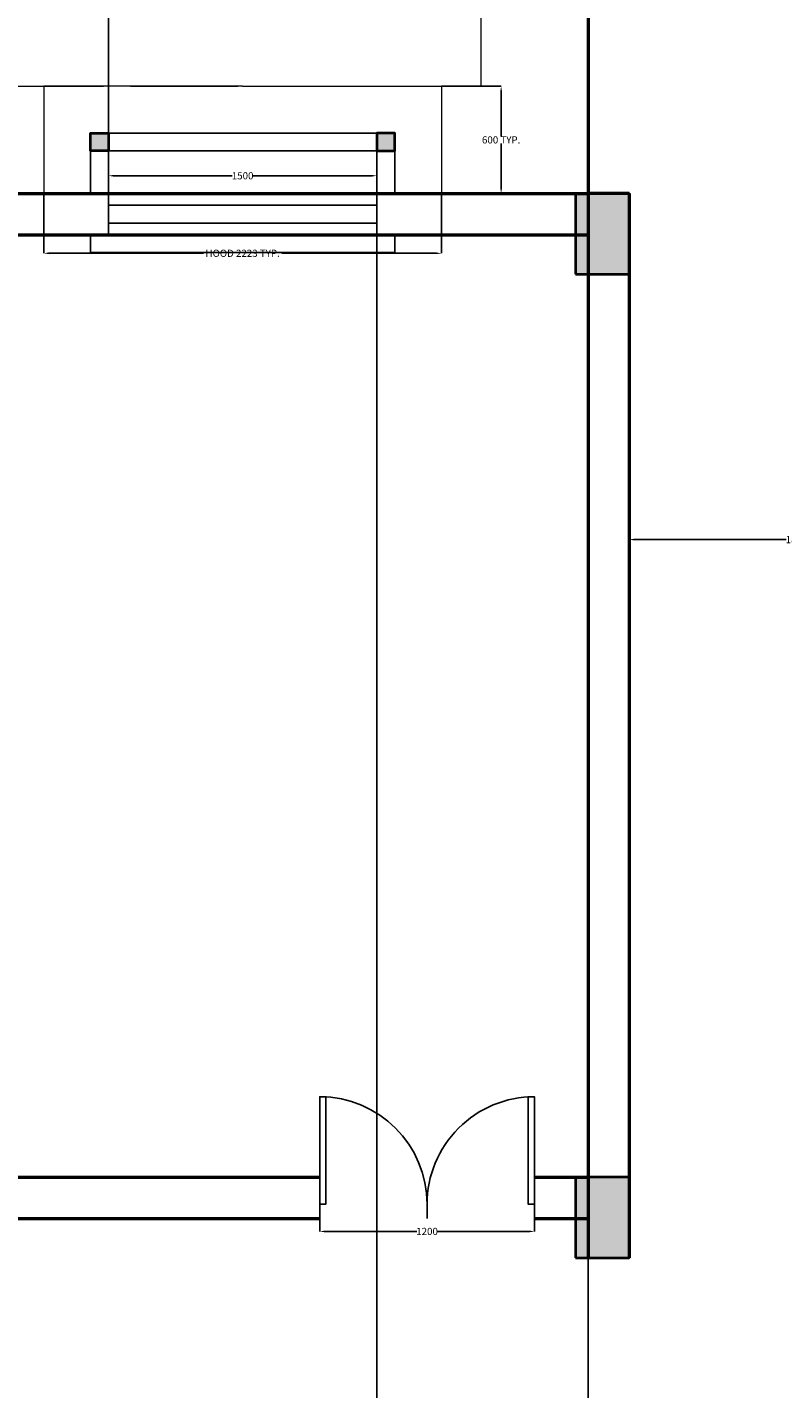
# Model space of a CAD drawing. Units: millimetres. Extents: x -17156 to 39375, y -45872 to -24892.
# Tile 8 of 12: x 1128 to 5351, y -41514 to -33909. Entities that reach past the tile are written whole.
import ezdxf

# ---------------------------------------------------------------- set-up
doc = ezdxf.new("R2010")
doc.units = ezdxf.units.MM
doc.header["$MEASUREMENT"] = 0
doc.linetypes.add('ACAD_ISO02W100', pattern=[15, 12, -3])
for name, color, linetype, lineweight in [('A-ANNO-DIMS', 2, 'Continuous', 18), ('A-COLS', 7, 'Continuous', 40), ('A-ROOF', 8, 'Continuous', 18), ('A-ROOF-OVHD', 8, 'ACAD_ISO02W100', 18), ('DOORS', 6, 'Continuous', 25), ('WALLS', 5, 'Continuous', 50), ('WINDOW', 240, 'Continuous', 25)]:
    doc.layers.add(name, color=color, linetype=linetype, lineweight=lineweight)
doc.layers.add('A-COLS-PATT', color=114, linetype='Continuous', lineweight=13, true_color=0x139b48)
doc.styles.get("Standard").update_dxf_attribs({"font": 'arial.ttf'})
doc.dimstyles.get("Standard").update_dxf_attribs({"dimtxt": 40, "dimasz": 30.18, "dimexe": 0, "dimexo": 0.0625, "dimgap": 0.09, "dimtad": 0, "dimtih": 1, "dimtoh": 1, "dimdec": 0, "dimzin": 0, "dimdsep": 46, "dimtxsty": 'Standard', "dimcen": 0.09, "dimadec": 0, "dimazin": 0, "dimtfac": 1, "dimtdec": 0, "dimtofl": 0, "dimtmove": 0, "dimatfit": 3, "dimfxl": 1, "dimtolj": 1, "dimtzin": 0, "dimarcsym": 0})

# ---------------------------------------------------------------- blocks, each defined once
blk = doc.blocks.new('*U7')
for p, q in [((0, 0), (0, 100)), ((750, 0), (750, 100))]:
    blk.add_line(p, q)
blk.add_lwpolyline([(0, 0), (0, -750), (43.75, -750), (43.75, 0)], close=True)
blk.add_arc((0, 0), 750, 270, 0)
blk = doc.blocks.new('*D102')
at = {"layer": 'A-ANNO-DIMS', "color": 0, "lineweight": -2, "transparency": 16777216}
for p, q in [((1581.8, -34837.8), (1581.8, -34738.2)), ((1612, -34738.2), (2274, -34738.2)), ((3051.7, -34738.2), (2389.7, -34738.2)), ((3081.8, -34837.8), (3081.8, -34738.2))]:
    blk.add_line(p, q, dxfattribs=at)
at = {"layer": 'A-ANNO-DIMS', "color": 0, "lineweight": 100, "transparency": 16777216}
for points in [[(1612, -34733.2), (1612, -34743.2), (1581.8, -34738.2)], [(3051.7, -34733.2), (3051.7, -34743.2), (3081.8, -34738.2)]]:
    blk.add_solid(points, dxfattribs=at)
at = {"layer": 'Defpoints', "color": 0, "lineweight": 100, "transparency": 16777216}
for p in [(3081.8, -34738.2), (1581.8, -34837.8), (3081.8, -34837.8)]:
    blk.add_point(p, dxfattribs=at)
at = {"layer": 'A-ANNO-DIMS', "color": 0, "transparency": 16777216, "insert": (2331.8, -34738.2), "char_height": 40, "attachment_point": 5}
blk.add_mtext('\\A1;1500', dxfattribs=at)
blk = doc.blocks.new('*D108')
at = {"layer": 'A-ANNO-DIMS', "color": 0, "lineweight": -2, "transparency": 16777216}
for p, q in [((4492.7, -36770.5), (4492.7, -36770.6)), ((4522.8, -36770.6), (5369.8, -36770.6)), ((6332.5, -36770.6), (5485.5, -36770.6)), ((6362.7, -36770.5), (6362.7, -36770.6))]:
    blk.add_line(p, q, dxfattribs=at)
at = {"layer": 'A-ANNO-DIMS', "color": 0, "lineweight": 100, "transparency": 16777216}
for points in [[(4522.8, -36765.6), (4522.8, -36775.6), (4492.7, -36770.6)], [(6332.5, -36765.6), (6332.5, -36775.6), (6362.7, -36770.6)]]:
    blk.add_solid(points, dxfattribs=at)
at = {"layer": 'Defpoints', "color": 0, "lineweight": 100, "transparency": 16777216}
for p in [(4492.7, -36770.6), (6362.7, -36770.6), (6362.7, -36770.6)]:
    blk.add_point(p, dxfattribs=at)
at = {"layer": 'A-ANNO-DIMS', "color": 0, "transparency": 16777216, "insert": (5427.7, -36770.6), "char_height": 40, "attachment_point": 5}
blk.add_mtext('\\A1;1870', dxfattribs=at)
blk = doc.blocks.new('*D109')
at = {"layer": 'A-ANNO-DIMS', "color": 0, "lineweight": -2, "transparency": 16777216}
for p, q in [((2762.7, -40562.9), (2762.7, -40635.1)), ((3962.7, -40562.9), (3962.7, -40635.1)), ((2792.8, -40635.1), (3304.8, -40635.1)), ((3932.5, -40635.1), (3420.5, -40635.1))]:
    blk.add_line(p, q, dxfattribs=at)
at = {"layer": 'A-ANNO-DIMS', "color": 0, "lineweight": 100, "transparency": 16777216}
for points in [[(2792.8, -40630.1), (2792.8, -40640.2), (2762.7, -40635.1)], [(3932.5, -40630.1), (3932.5, -40640.2), (3962.7, -40635.1)]]:
    blk.add_solid(points, dxfattribs=at)
at = {"layer": 'Defpoints', "color": 0, "lineweight": 100, "transparency": 16777216}
for p in [(2762.7, -40562.8), (3962.7, -40562.8), (3962.7, -40635.1)]:
    blk.add_point(p, dxfattribs=at)
at = {"layer": 'A-ANNO-DIMS', "color": 0, "transparency": 16777216, "insert": (3362.7, -40635.1), "char_height": 40, "attachment_point": 5}
blk.add_mtext('\\A1;1200', dxfattribs=at)
blk = doc.blocks.new('WIN-COURTYARD-1500')
for p, q in [((1600, 668), (100, 668)), ((0, 568), (0, 330)), ((100, 568), (100, 330)), ((1600, 568), (100, 568)), ((1600, 568), (1600, 330)), ((1700, 568), (1700, 330)), ((100, 330), (100, 100)), ((100, 330), (1600, 330)), ((1600, 330), (1600, 100)), ((100, 265), (1600, 265)), ((100, 165), (1600, 165)), ((0, 100), (0, 0)), ((0, 100), (100, 100)), ((100, 100), (1700, 100)), ((1700, 0), (1700, 100)), ((0, 0), (1700, 0))]:
    blk.add_line(p, q)
blk = doc.blocks.new('COL-450x300')
h = blk.add_hatch(color=256)
h.dxf.hatch_style = 1
h.paths.add_polyline_path([(0, 300), (0, 0), (450, 0), (450, 300)])
blk.add_lwpolyline([(0, 300), (0, 0), (450, 0), (450, 300)], close=True)
blk = doc.blocks.new('WINDOW-HOOD-2223x600')
for p, q in [((0, 600), (0, 0)), ((1111.5, 600), (0, 600)), ((1111.5, 600), (2223, 600)), ((2223, 600), (2223, 0))]:
    blk.add_line(p, q)
blk = doc.blocks.new('*D138')
at = {"layer": 'A-ANNO-DIMS', "color": 0, "lineweight": -2, "transparency": 16777216}
for p, q in [((1220.3, -34837.9), (1220.3, -35171.3)), ((3443.3, -34837.9), (3443.3, -35171.3)), ((1250.5, -35171.3), (2112.8, -35171.3)), ((3413.2, -35171.3), (2550.9, -35171.3))]:
    blk.add_line(p, q, dxfattribs=at)
at = {"layer": 'A-ANNO-DIMS', "color": 0, "lineweight": 100, "transparency": 16777216}
for points in [[(1250.5, -35166.3), (1250.5, -35176.3), (1220.3, -35171.3)], [(3413.2, -35166.3), (3413.2, -35176.3), (3443.3, -35171.3)]]:
    blk.add_solid(points, dxfattribs=at)
at = {"layer": 'Defpoints', "color": 0, "lineweight": 100, "transparency": 16777216}
for p in [(1220.3, -34837.8), (3443.3, -34837.8), (3443.3, -35171.3)]:
    blk.add_point(p, dxfattribs=at)
at = {"layer": 'A-ANNO-DIMS', "color": 0, "transparency": 16777216, "insert": (2331.8, -35171.3), "char_height": 40, "attachment_point": 5}
blk.add_mtext('\\A1;HOOD 2223 TYP.', dxfattribs=at)
blk = doc.blocks.new('*D139')
at = {"layer": 'A-ANNO-DIMS', "color": 0, "lineweight": -2, "transparency": 16777216}
for p, q in [((3443.4, -34237.8), (3776.8, -34237.8)), ((3776.8, -34268), (3776.8, -34517.3)), ((3776.8, -34807.7), (3776.8, -34558.4)), ((3443.4, -34837.8), (3776.8, -34837.8))]:
    blk.add_line(p, q, dxfattribs=at)
at = {"layer": 'A-ANNO-DIMS', "color": 0, "lineweight": 100, "transparency": 16777216}
for points in [[(3771.8, -34268), (3781.8, -34268), (3776.8, -34237.8)], [(3771.8, -34807.7), (3781.8, -34807.7), (3776.8, -34837.8)]]:
    blk.add_solid(points, dxfattribs=at)
at = {"layer": 'Defpoints', "color": 0, "lineweight": 100, "transparency": 16777216}
for p in [(3443.3, -34237.8), (3776.8, -34237.8), (3443.3, -34837.8)]:
    blk.add_point(p, dxfattribs=at)
at = {"layer": 'A-ANNO-DIMS', "color": 0, "transparency": 16777216, "insert": (3776.8, -34537.8), "char_height": 40, "attachment_point": 5}
blk.add_mtext('\\A1;600 TYP.', dxfattribs=at)
blk = doc.blocks.new('*D149')
at = {"layer": 'A-ANNO-DIMS', "color": 0, "lineweight": -2, "transparency": 16777216}
for p, q in [((-262.3, -34837.8), (-262.3, -25564.8)), ((-232.1, -25564.8), (601.9, -25564.8)), ((1551.7, -25564.8), (717.6, -25564.8)), ((1581.8, -34837.8), (1581.8, -25564.8))]:
    blk.add_line(p, q, dxfattribs=at)
at = {"layer": 'A-ANNO-DIMS', "color": 0, "lineweight": 100, "transparency": 16777216}
for points in [[(-232.1, -25559.8), (-232.1, -25569.9), (-262.3, -25564.8)], [(1551.7, -25559.8), (1551.7, -25569.9), (1581.8, -25564.8)]]:
    blk.add_solid(points, dxfattribs=at)
at = {"layer": 'Defpoints', "color": 0, "lineweight": 100, "transparency": 16777216}
for p in [(1581.8, -25564.8), (-262.3, -34837.8), (1581.8, -34837.8)]:
    blk.add_point(p, dxfattribs=at)
at = {"layer": 'A-ANNO-DIMS', "color": 0, "transparency": 16777216, "insert": (659.8, -25564.8), "char_height": 40, "attachment_point": 5}
blk.add_mtext('\\A1;1844', dxfattribs=at)
blk = doc.blocks.new('*D150')
at = {"layer": 'A-ANNO-DIMS', "color": 0, "lineweight": -2, "transparency": 16777216}
for p, q in [((3081.8, -35067.9), (3081.8, -45845.8)), ((4262.7, -35067.9), (4262.7, -45845.8)), ((3112, -45845.8), (3591, -45845.8)), ((4232.5, -45845.8), (3753.5, -45845.8))]:
    blk.add_line(p, q, dxfattribs=at)
at = {"layer": 'A-ANNO-DIMS', "color": 0, "lineweight": 100, "transparency": 16777216}
for points in [[(3112, -45840.8), (3112, -45850.9), (3081.8, -45845.8)], [(4232.5, -45840.8), (4232.5, -45850.9), (4262.7, -45845.8)]]:
    blk.add_solid(points, dxfattribs=at)
at = {"layer": 'Defpoints', "color": 0, "lineweight": 100, "transparency": 16777216}
for p in [(3081.8, -35067.8), (4262.7, -35067.8), (4262.7, -45845.8)]:
    blk.add_point(p, dxfattribs=at)
at = {"layer": 'A-ANNO-DIMS', "color": 0, "transparency": 16777216, "insert": (3672.2, -45845.8), "char_height": 40, "attachment_point": 5}
blk.add_mtext('\\A1;1180.8', dxfattribs=at)

msp = doc.modelspace()

# ---------------------------------------------------------------- hatches: boundary and pattern name
at = {"layer": 'A-COLS-PATT'}
h = msp.add_hatch(color=256, dxfattribs=at)
h.dxf.hatch_style = 1
h.paths.add_polyline_path([(-6007.35, -42547.85, 1), (-6237.35, -42547.85, 1)])
h.paths.add_polyline_path([(-2699.35, -42547.85, 1), (-2469.35, -42547.85, 1)])
h.paths.add_polyline_path([(424.65, -42547.85, 1), (654.65, -42547.85, 1)])
h.paths.add_polyline_path([(3997.65, -42547.85, 1), (4227.65, -42547.85, 1)])
h.paths.add_polyline_path([(1581.84, -34499.85), (1481.84, -34499.85), (1481.84, -34599.85), (1581.84, -34599.85)])
h.paths.add_polyline_path([(3181.84, -34499.85), (3081.84, -34499.85), (3081.84, -34599.85), (3181.84, -34599.85)])
h.paths.add_polyline_path([(-162.32, -34499.85), (-262.32, -34499.85), (-262.32, -34599.85), (-162.32, -34599.85)])
h.paths.add_polyline_path([(-1762.32, -34499.85), (-1862.32, -34499.85), (-1862.32, -34599.85), (-1762.32, -34599.85)])
h.paths.add_polyline_path([(-3445.85, -34499.85), (-3545.85, -34499.85), (-3545.85, -34599.85), (-3445.85, -34599.85)])
h.paths.add_polyline_path([(-5045.85, -34499.85), (-5145.85, -34499.85), (-5145.85, -34599.85), (-5045.85, -34599.85)])

# ---------------------------------------------------------------- linework, layer by layer
at = {"layer": 'A-COLS'}
for points in [[(1581.84, -34599.85), (1481.84, -34599.85), (1481.84, -34499.85), (1581.84, -34499.85)], [(3081.84, -34599.85), (3181.84, -34599.85), (3181.84, -34499.85), (3081.84, -34499.85)]]:
    msp.add_lwpolyline(points, close=True, dxfattribs=at)
at = {"layer": 'A-ROOF-OVHD', "ltscale": 50}
for p in [(3662.65, -31607.85), (-3545.85, -34237.85)]:
    msp.add_line(p, (3662.65, -34237.85), dxfattribs=at)
at = {"layer": 'DOORS'}
msp.add_line((3962.65, -39882.85), (3962.65, -40562.85), dxfattribs=at)
at = {"layer": 'WALLS'}
for p, q in [((4262.65, -31607.85), (4262.65, -34837.85)), ((-3545.85, -34837.85), (4262.65, -34837.85)), ((4262.65, -34837.85), (4262.65, -40782.85)), ((4492.65, -34837.85), (4262.65, -34837.85)), ((4492.65, -34837.85), (4492.65, -40782.85)), ((-3445.85, -35067.85), (4262.65, -35067.85)), ((-4737.35, -40332.85), (2762.65, -40332.85)), ((3962.65, -40332.85), (4262.65, -40332.85)), ((-122.35, -40562.85), (2762.65, -40562.85)), ((3962.65, -40562.85), (4262.65, -40562.85))]:
    msp.add_line(p, q, dxfattribs=at)

# ---------------------------------------------------------------- block references
at = {"layer": 'A-COLS', "rotation": 90.00000000000124}
for p in [(4492.65, -35287.85), (4492.65, -40782.85)]:
    msp.add_blockref('COL-450x300', p, dxfattribs=at)
at = {"layer": 'A-ROOF'}
msp.add_blockref('WINDOW-HOOD-2223x600', (1220.34, -34837.85), dxfattribs=at)
at = {"layer": 'DOORS', "yscale": 0.8, "zscale": 0.8, "rotation": 180}
for p, xscale in [((2762.65, -40482.85), -0.8), ((3962.65, -40482.85), 0.8)]:
    msp.add_blockref('*U7', p, dxfattribs=dict(at, xscale=xscale))
at = {"layer": 'WINDOW'}
msp.add_blockref('WIN-COURTYARD-1500', (1481.84, -35167.85), dxfattribs=at)

# ---------------------------------------------------------------- dimensions: what is measured, and where the dimension line sits
at = {"layer": 'A-ANNO-DIMS'}
for base, p1, p2, override, picture, middle in [((1581.84, -25564.85), (-262.32, -34837.85), (1581.84, -34837.85), {"dimdec": 0, "dimlfac": 1, "dimrnd": 0, "dimzin": 0, "dimdsep": 46, "dimlunit": 2}, '*D149', (659.76, -25564.85)), ((3081.84, -34738.22), (1581.84, -34837.85), (3081.84, -34837.85), {"dimclrd": 0, "dimclre": 0, "dimclrt": 0}, '*D102', (2331.84, -34738.22)), ((4262.65, -45845.85), (3081.84, -35067.85), (4262.65, -35067.85), {"dimdec": 1, "dimlfac": 1, "dimrnd": 0, "dimzin": 0, "dimdsep": 46, "dimlunit": 2}, '*D150', (3672.24, -45845.85)), ((6362.65, -36770.59), (4492.65, -36770.59), (6362.65, -36770.59), {"dimclrd": 0, "dimclre": 0, "dimclrt": 0}, '*D108', (5427.65, -36770.59)), ((3962.65, -40635.15), (2762.65, -40562.85), (3962.65, -40562.85), {"dimclrd": 0, "dimclre": 0, "dimclrt": 0}, '*D109', (3362.65, -40635.15))]:
    dim = msp.add_linear_dim(base=base, p1=p1, p2=p2, dimstyle='Standard', override=override, dxfattribs=at)
    dim.commit()
    dim.dimension.update_dxf_attribs({"geometry": picture, "text_midpoint": middle})
dim = msp.add_linear_dim(base=(3776.79, -34237.85), p1=(3443.34, -34837.85), p2=(3443.34, -34237.85), angle=90, text='<> TYP.', dimstyle='Standard', override={"dimdec": 0, "dimlfac": 1, "dimrnd": 0, "dimzin": 0, "dimdsep": 46, "dimlunit": 2}, dxfattribs=at)
dim.commit()
dim.dimension.update_dxf_attribs({"geometry": '*D139', "text_midpoint": (3776.79, -34537.85)})
dim = msp.add_linear_dim(base=(3443.34, -35171.3), p1=(1220.34, -34837.85), p2=(3443.34, -34837.85), text='HOOD <> TYP.', dimstyle='Standard', override={"dimdec": 0, "dimlfac": 1, "dimrnd": 0, "dimzin": 0, "dimdsep": 46, "dimlunit": 2}, dxfattribs=at)
dim.commit()
dim.dimension.update_dxf_attribs({"geometry": '*D138', "text_midpoint": (2331.84, -35171.3)})

doc.saveas('drawing.dxf')
